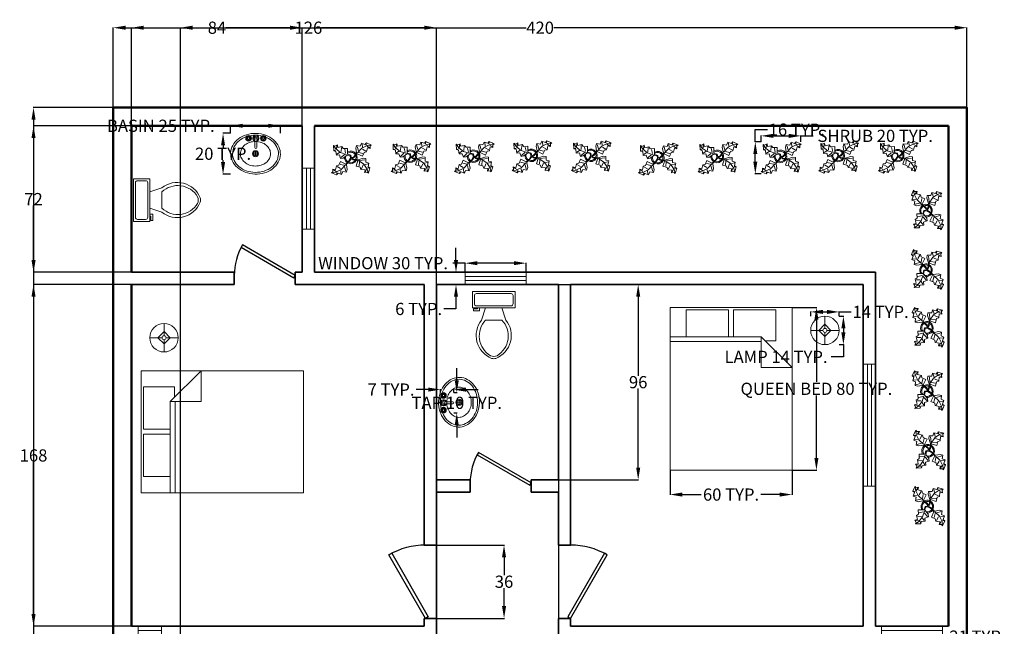
# Model space of a CAD drawing. Units: inches. Extents: x 823 to 1335, y 207 to 1074.
# Tile 6 of 6: x 823 to 1308, y 776 to 1074. Entities that reach past the tile are written whole.
import ezdxf

# ---------------------------------------------------------------- set-up
doc = ezdxf.new("R2010")
doc.units = ezdxf.units.IN
doc.header["$MEASUREMENT"] = 0
for name, color, linetype, lineweight in [('A-ANNO-DIMS', 2, 'Continuous', 18), ('doors', 51, 'Continuous', 25), ('furniture', 21, 'Continuous', 18), ('inner wall', 102, 'Continuous', 35), ('L-PLNT', 90, 'Continuous', 13), ('outer wall', 105, 'Continuous', 50), ('sanitary', 131, 'Continuous', 18), ('windows', 211, 'Continuous', 18)]:
    doc.layers.add(name, color=color, linetype=linetype, lineweight=lineweight)
doc.styles.get("Standard").update_dxf_attribs({"font": 'arial.ttf'})
doc.dimstyles.get("Standard").update_dxf_attribs({"dimtxt": 6, "dimasz": 6, "dimexe": 0.18, "dimexo": 0.0625, "dimgap": 0.09, "dimtad": 0, "dimtih": 1, "dimtoh": 1, "dimdec": 0, "dimzin": 0, "dimdsep": 46, "dimlunit": 3, "dimtxsty": 'Standard', "dimcen": 0.09, "dimadec": 0, "dimazin": 0, "dimtfac": 1, "dimtdec": 0, "dimtofl": 0, "dimtmove": 0, "dimatfit": 3, "dimfxl": 1, "dimtolj": 1, "dimtzin": 0, "dimarcsym": 0})

# ---------------------------------------------------------------- blocks, each defined once
blk = doc.blocks.new('*U3')
for p, q in [((0, 0), (0, 6)), ((40, 0), (40, 6))]:
    blk.add_line(p, q)
blk.add_lwpolyline([(0, 0), (34.64, -20), (35.52, -18.48), (0.87, 1.52)], close=True)
blk.add_arc((0, 0), 40, 330, 0)
blk = doc.blocks.new('*U2')
for p, q in [((0, 0), (0, -6)), ((40, 0), (40, -6))]:
    blk.add_line(p, q)
blk.add_lwpolyline([(0, 0), (34.64, 20), (35.52, 18.48), (0.87, -1.52)], close=True)
blk.add_arc((0, 0), 40, 0, 30)
blk = doc.blocks.new('*U5')
for p, q in [((0, 0), (0, -6)), ((-40, 0), (-40, -6))]:
    blk.add_line(p, q)
blk.add_lwpolyline([(0, 0), (-34.64, 20), (-35.52, 18.48), (-0.88, -1.52)], close=True)
blk.add_arc((0, 0), 40, 150, 180)
blk = doc.blocks.new('Bed - Queen')
for p, q in [((0, -80.00003), (0, 0)), ((0, 0), (59.99999, 0)), ((59.99999, 0), (59.99999, -80.00003)), ((7.99999, -1.2), (28.79998, -1.2)), ((7.99999, -14.4), (7.99999, -1.2)), ((28.79998, -1.2), (28.79998, -14.4)), ((31.19999, -1.2), (51.99999, -1.2)), ((31.19999, -14.4), (31.19999, -1.2)), ((51.99999, -1.2), (51.99999, -16.4)), ((0, -14.4), (44.8, -14.4)), ((59.99999, -29.6), (44.8, -14.4)), ((44.8, -14.4), (44.8, -29.6)), ((44.8, -16.8), (0, -16.8)), ((51.99999, -16.4), (46.79936, -16.4)), ((44.8, -29.6), (59.99999, -29.6)), ((59.99999, -80.00003), (0, -80.00003))]:
    blk.add_line(p, q)
blk = doc.blocks.new('Lamp - Table')
for p, q in [((0, 7), (0, 1)), ((-1, 0), (-7, 0)), ((0, 3), (-3, 0)), ((-3, 0), (0, -3)), ((3, 0), (0, 3)), ((0, -3), (3, 0)), ((1, 0), (7, 0)), ((0, -1), (0, -7))]:
    blk.add_line(p, q)
for radius in [7, 1]:
    blk.add_circle((0, 0), radius)
blk = doc.blocks.new('Sink - Oval top')
for p, q in [((-1, 0), (1, 0)), ((0, 1), (0, -1))]:
    blk.add_line(p, q)
for points in [[(-12.23, 0.39, 0.117634), (-11.46, -3.36, 0.104469), (-8.88, -6.8, 0.090016), (-5.08, -9.07, 0.08192), (-0.32, -10.02, 0.08192), (4.49, -9.38, 0.090016), (8.42, -7.36, 0.104469), (11.22, -4.09, 0.117634), (12.23, -0.39, 0.117634), (11.46, 3.36, 0.104469), (8.88, 6.8, 0.090016), (5.08, 9.07, 0.08192), (0.32, 10.02, 0.08192), (-4.49, 9.38, 0.090016), (-8.42, 7.36, 0.104469), (-11.22, 4.09, 0.117634)], [(-11.29, 0.16, 0.118622), (-10.52, -3.25, 0.104678), (-8.07, -6.36, 0.089562), (-4.54, -8.37, 0.081185), (-0.13, -9.15, 0.081185), (4.3, -8.49, 0.089562), (7.89, -6.58, 0.104678), (10.42, -3.55, 0.118622), (11.29, -0.16, 0.118622), (10.52, 3.25, 0.104678), (8.07, 6.36, 0.089562), (4.54, 8.37, 0.081185), (0.13, 9.15, 0.081185), (-4.3, 8.49, 0.089562), (-7.89, 6.58, 0.104678), (-10.42, 3.55, 0.118622)], [(-7.42, 0.08, 0.118283), (-6.91, -2.17, 0.104607), (-5.29, -4.21, 0.089718), (-2.97, -5.53, 0.081436), (-0.07, -6.04, 0.081436), (2.84, -5.59, 0.089718), (5.2, -4.33, 0.104607), (6.86, -2.32, 0.118283), (7.42, -0.08, 0.118283), (6.91, 2.17, 0.104607), (5.29, 4.21, 0.089718), (2.97, 5.53, 0.081436), (0.07, 6.04, 0.081436), (-2.84, 5.59, 0.089718), (-5.2, 4.33, 0.104607), (-6.86, 2.32, 0.118283)]]:
    blk.add_lwpolyline(points, format="xyb", close=True)
for radius in [1.5, 1]:
    blk.add_circle((0, 0), radius)
blk = doc.blocks.new('Faucet - Bathroom top')
for p, q in [((-4.107, 0.125), (-4.375, 0.125)), ((-3.75, 0.4788), (-3.75, 0.75)), ((-3.5, 0.482), (-3.5, 0.75)), ((-3.1461, 0.125), (-2.875, 0.125)), ((3.143, 0.125), (2.875, 0.125)), ((3.5, 0.4788), (3.5, 0.75)), ((3.75, 0.482), (3.75, 0.75)), ((4.1039, 0.125), (4.375, 0.125)), ((-4.1039, -0.125), (-4.375, -0.125)), ((-3.75, -0.4821), (-3.75, -0.75)), ((-3.5, -0.4789), (-3.5, -0.75)), ((-3.143, -0.125), (-2.875, -0.125)), ((-0.5, -0.8639), (-0.5, -4.5)), ((0.5, -4.5), (0.5, -0.8631)), ((3.1461, -0.125), (2.875, -0.125)), ((3.5, -0.4821), (3.5, -0.75)), ((3.75, -0.4789), (3.75, -0.75)), ((4.107, -0.125), (4.375, -0.125))]:
    blk.add_line(p, q)
for centre, radius in [((-3.625, 0), 1.375), ((-4.625, 0), 0.2795), ((-3.625, 0), 0.5), ((-3.625, 1), 0.2795), ((-2.625, 0), 0.2795), ((0, 0), 0.5), ((3.625, 0), 1.375), ((2.625, 0), 0.2795), ((3.625, 0), 0.5), ((3.625, 1), 0.2795), ((4.625, 0), 0.2795), ((-3.625, -1), 0.2795), ((3.625, -1), 0.2795)]:
    blk.add_circle(centre, radius)
for centre, radius, start, end in [((-3.625, 0), 1, 105.2407, 164.2093), ((-3.625, 0), 1, 16.44125, 74.07887), ((0, 0), 1.5, 289.6514, 250.3603), ((0, 0), 1, 300.3431, 239.7554), ((3.625, 0), 1, 106.12, 164.0884), ((3.625, 0), 1, 16.23422, 73.90469), ((-3.625, 0), 1, 196.2342, 253.9047), ((-3.625, 0), 1, 286.12, 344.0884), ((0, -4.5), 0.5, 180, 0), ((3.625, 0), 1, 196.4413, 254.0789), ((3.625, 0), 1, 285.2407, 344.2093)]:
    blk.add_arc(centre, radius, start, end)
blk = doc.blocks.new('Toilet - top')
for p, q in [((9.5, -6), (9.5, -2)), ((-10, -8.5), (-8, -8.5)), ((-10, -9.5), (-10, -8.5)), ((-7, -9.5), (-10, -9.5)), ((-8, -8.5), (-8, -8)), ((-7, -8), (-7, -9.5)), ((-4, -8), (-6, -14)), ((4, -8), (6, -14)), ((4, -14), (-4, -14))]:
    blk.add_line(p, q)
blk.add_lwpolyline([(10.5, -8), (10.5, 0), (-10.5, 0), (-10.5, -8)], close=True)
for points in [[(-9.5, -2), (-9.5, -6)], [(8.5, -1), (-8.5, -1)], [(-8.5, -7), (8.5, -7)]]:
    blk.add_lwpolyline(points)
for centre, radius, start, end in [((-8.62, -1.88), 0.884, 81.8699, 188.1301), ((8.62, -1.88), 0.884, 351.8699, 98.1301), ((-8.62, -6.12), 0.884, 171.8699, 278.1301), ((8.62, -6.12), 0.884, 261.8699, 8.1301), ((3.52, -21.58), 12.17, 141.4691, 247.9714), ((4.2, -21.82), 11.33, 136.3677, 238.9468), ((-3.52, -21.58), 12.17, 292.0284, 38.5307), ((-4.2, -21.82), 11.33, 301.053, 43.6321), ((0, -27.88), 4, 245.7318, 294.2682), ((0, -29), 4, 254.8605, 285.1395)]:
    blk.add_arc(centre, radius, start, end)
blk = doc.blocks.new('Plant - Rubber or Philodendron')
for p, q in [((-16.2005, 11.4774), (-13.9899, 8.1064)), ((-16.2005, 11.4774), (-14.8639, 10.7964)), ((-16.0159, 6.3329), (-16.2005, 11.4774)), ((-14.8639, 10.7964), (-12.6195, 11.8975)), ((-13.3174, 8.325), (-13.0735, 11.0065)), ((-12.6195, 11.8975), (-12.1909, 9.4345)), ((-12.1909, 9.4345), (-8.3829, 10.3)), ((-8.8369, 9.409), (-9.0894, 5.6095)), ((-8.3829, 10.3), (-7.0549, 8.501)), ((4.6914, 8.8812), (5.3859, 11.2828)), ((5.3859, 11.2828), (8.8871, 10.7908)), ((5.9878, 10.4842), (7.1971, 6.3869)), ((8.8871, 10.7908), (9.9809, 13.4933)), ((9.9809, 13.4933), (13.3837, 12.301)), ((15.3859, 11.3055), (10.3916, 8.7942)), ((10.5828, 12.6946), (10.8893, 9.7953)), ((13.3837, 12.301), (14.68, 13.9039)), ((14.5816, 13.2037), (14.3848, 11.8033)), ((14.68, 13.9039), (19.3848, 11.8146)), ((15.2875, 10.6053), (17.5907, 9.2105)), ((19.3848, 11.8146), (15.3859, 11.3055)), ((19.3848, 11.8146), (18.1868, 10.9119)), ((18.1868, 10.9119), (18.1925, 8.4119)), ((-14.0069, 5.8704), (-16.0159, 6.3329)), ((-15.3434, 6.5514), (-13.9984, 6.9884)), ((-13.5868, 2.2894), (-14.0069, 5.8704)), ((-13.9899, 8.1064), (-9.5434, 4.7185)), ((-10.6784, 2.491), (-13.5868, 2.2894)), ((-13.1329, 3.1804), (-10.6614, 4.727)), ((-9.5858, -0.8715), (-10.6784, 2.491)), ((-9.5434, 4.7185), (-4.1917, 2.9888)), ((-9.1318, 0.0195), (-5.9793, 2.9025)), ((-7.1228, -0.443), (-3.5248, 2.2131)), ((-7.0549, 8.501), (-3.0284, 8.6941)), ((-4.8529, 4.012), (-5.7184, 7.82)), ((-3.5248, 2.2131), (-3.3011, 2.4355)), ((-3.3011, 2.4355), (-0.5306, 1.7947)), ((-3.0284, 8.6941), (-3.0709, 3.1041)), ((-3.0709, 3.1041), (0.0797, 2.3163)), ((-0.5306, 1.7947), (-0.2255, -0.5527)), ((-0.5306, 1.7947), (-0.5306, 1.7947)), ((0.0797, 2.3163), (0.4866, -0.031)), ((0.4866, -0.031), (2.1141, 0.2298)), ((2.1141, 0.2298), (5.4346, 3.9146)), ((6.1032, 3.6844), (2.8262, -0.031)), ((4.6914, 8.8812), (5.5014, 4.4831)), ((5.4346, 3.9146), (5.5014, 4.4831)), ((11.1089, 1.1958), (6.1032, 3.6844)), ((10.3916, 8.7942), (6.2847, 4.4028)), ((7.7005, 4.8881), (11.5025, 3.9967)), ((14.2977, 6.1031), (10.9934, 7.9956)), ((12.7005, 4.8994), (11.1089, 1.1958)), ((14.8995, 5.3044), (12.7005, 4.8994)), ((15.7909, 9.1065), (14.8995, 5.3044)), ((18.1925, 8.4119), (15.7909, 9.1065)), ((-14.4141, -11.4699), (-13.5228, -7.6679)), ((-13.5228, -7.6679), (-11.3237, -7.2629)), ((-12.921, -8.4665), (-9.6166, -10.359)), ((-11.3237, -7.2629), (-9.7321, -3.5593)), ((-6.3237, -7.2516), (-10.1257, -6.3602)), ((-9.7321, -3.5593), (-4.7264, -6.0479)), ((-7.1228, -0.443), (-9.5858, -0.8715)), ((-9.0148, -11.1577), (-4.9047, -6.8122)), ((-4.611, -12.8477), (-5.8203, -8.7504)), ((-2.019, -3.6148), (-4.7264, -6.0479)), ((-4.1246, -6.8466), (-4.0579, -6.2781)), ((-3.3146, -11.2447), (-4.1246, -6.8466)), ((-4.0579, -6.2781), (-0.9375, -3.1608)), ((-2.019, -3.6148), (-0.2255, -0.5527)), ((-0.9375, -3.1608), (0.5883, -0.8135)), ((0.5883, -0.8135), (2.2447, -2.0916)), ((2.8262, -0.031), (1.3003, -0.5527)), ((1.3003, -0.5527), (2.4193, -1.4655)), ((2.2447, -2.0916), (6.7108, -2.6626)), ((2.4193, -1.4655), (6.895, -2.1175)), ((4.943, -7.9659), (6.7108, -2.6626)), ((8.8321, -9.0266), (4.943, -7.9659)), ((11.6605, -0.5413), (6.895, -2.1175)), ((12.3677, -6.1981), (7.219, -2.6772)), ((8.125, -4.0768), (7.7715, -7.9659)), ((8.3544, -2.7453), (13.1973, -2.1704)), ((9.5392, -11.1479), (8.8321, -9.0266)), ((10.2463, -10.4408), (11.6605, -6.9053)), ((11.6605, -0.5413), (14.1354, -0.8948)), ((15.5496, -10.7943), (12.3677, -6.1981)), ((16.2567, -5.8446), (13.4283, -6.5517)), ((14.1354, -0.8948), (14.1354, -4.4304)), ((14.1354, -4.4304), (16.9638, -5.1375)), ((16.9638, -5.1375), (16.2567, -8.673)), ((16.2567, -8.673), (18.0245, -9.7337)), ((-18.008, -14.1781), (-16.8101, -13.2754)), ((-18.008, -14.1781), (-14.0091, -13.669)), ((-13.3032, -16.2674), (-18.008, -14.1781)), ((-16.8157, -10.7754), (-14.4141, -11.4699)), ((-16.8101, -13.2754), (-16.8157, -10.7754)), ((-13.9107, -12.9688), (-16.2139, -11.574)), ((-14.0091, -13.669), (-9.0148, -11.1577)), ((-12.0069, -14.6645), (-13.3032, -16.2674)), ((-13.2048, -15.5672), (-13.008, -14.1668)), ((-8.6042, -15.8568), (-12.0069, -14.6645)), ((-9.206, -15.0581), (-9.5126, -12.1588)), ((-7.5103, -13.1543), (-8.6042, -15.8568)), ((-4.0092, -13.6463), (-7.5103, -13.1543)), ((-3.3146, -11.2447), (-4.0092, -13.6463)), ((13.4283, -11.5015), (9.5392, -11.1479)), ((13.0748, -13.9763), (13.4283, -11.5015)), ((15.5496, -13.6228), (13.0748, -13.9763)), ((14.8425, -10.7943), (13.7819, -13.2692)), ((16.6103, -14.6834), (15.5496, -10.7943)), ((16.6103, -14.6834), (15.5496, -13.6228)), ((17.3174, -9.7337), (15.9032, -9.7337)), ((18.0245, -9.7337), (16.6103, -14.6834))]:
    blk.add_line(p, q)
for centre, radius, start, end in [((0.0308, 0.1664), 6, 178.6147, 235.1169), ((0.0308, 0.1664), 5, 168.1647, 238.6725), ((0, 0), 6.1275, 34.37569, 120.1028), ((-0.0601, -0.2075), 5.2461, 33.82192, 124.9414), ((-0.2664, 0.1682), 5.2775, 338.4094, 20.03007), ((-0.098, 0.1364), 6.1288, 341.2017, 26.09184), ((-0.0234, 0.3825), 6.1492, 242.5812, 331.2714), ((-0.1102, 0.4886), 5.2883, 247.3711, 327.472)]:
    blk.add_arc(centre, radius, start, end)
blk = doc.blocks.new('WIN-60IN')
for p, q in [((0, 0), (0, 60)), ((0, 60), (6, 60)), ((2, 0), (2, 60)), ((4, 60), (4, 0)), ((6, 60), (6, 0)), ((6, 0), (0, 0))]:
    blk.add_line(p, q)
blk = doc.blocks.new('WIN-30IN')
for p, q in [((0, 6), (30, 6)), ((0, 0), (0, 6)), ((30, 6), (30, 0)), ((0, 4), (30, 4)), ((30, 2), (0, 2)), ((30, 0), (0, 0))]:
    blk.add_line(p, q)
blk = doc.blocks.new('WIN-LIGHTWELL-NARROW')
for p, q in [((0, 6), (0, 0)), ((11.5, 6), (11.5, 0)), ((0, 4), (11.5, 4)), ((0, 2), (11.5, 2))]:
    blk.add_line(p, q)
blk = doc.blocks.new('*D26')
at = {"layer": 'A-ANNO-DIMS', "color": 0, "lineweight": -2, "transparency": 16777216}
for p, q in [((1203.26, 932.36), (1215.38, 932.36)), ((1215.2, 926.36), (1215.2, 895.74)), ((1215.2, 858.36), (1215.2, 888.99)), ((1203.26, 852.36), (1215.38, 852.36))]:
    blk.add_line(p, q, dxfattribs=at)
for points in [[(1214.2, 926.36), (1216.2, 926.36), (1215.2, 932.36)], [(1214.2, 858.36), (1216.2, 858.36), (1215.2, 852.36)]]:
    blk.add_solid(points, dxfattribs=at)
at = {"layer": 'Defpoints', "color": 0, "lineweight": -2, "transparency": 16777216}
for p in [(1203.2, 932.36), (1215.2, 932.36), (1203.2, 852.36)]:
    blk.add_point(p, dxfattribs=at)
at = {"layer": 'A-ANNO-DIMS', "color": 0, "transparency": 16777216, "insert": (1215.2, 892.36), "char_height": 6, "attachment_point": 5}
blk.add_mtext('\\A1;QUEEN BED 80 TYP.', dxfattribs=at)
blk = doc.blocks.new('*D27')
at = {"layer": 'A-ANNO-DIMS', "color": 0, "lineweight": -2, "transparency": 16777216}
for p, q in [((1143.2, 852.3), (1143.2, 840.18)), ((1203.2, 852.3), (1203.2, 840.18)), ((1149.2, 840.36), (1158.49, 840.36)), ((1197.2, 840.36), (1187.91, 840.36))]:
    blk.add_line(p, q, dxfattribs=at)
for points in [[(1149.2, 841.36), (1149.2, 839.36), (1143.2, 840.36)], [(1197.2, 841.36), (1197.2, 839.36), (1203.2, 840.36)]]:
    blk.add_solid(points, dxfattribs=at)
at = {"layer": 'Defpoints', "color": 0, "lineweight": -2, "transparency": 16777216}
for p in [(1143.2, 852.36), (1203.2, 852.36), (1203.2, 840.36)]:
    blk.add_point(p, dxfattribs=at)
at = {"layer": 'A-ANNO-DIMS', "color": 0, "transparency": 16777216, "insert": (1173.2, 840.36), "char_height": 6, "attachment_point": 5}
blk.add_mtext('\\A1;60 TYP.', dxfattribs=at)
blk = doc.blocks.new('*D28')
at = {"layer": 'A-ANNO-DIMS', "color": 0, "lineweight": -2, "transparency": 16777216}
for p, q in [((1226.44, 928.05), (1228.66, 928.05)), ((1228.48, 922.05), (1228.48, 920.05)), ((1226.44, 914.05), (1228.66, 914.05)), ((1228.48, 914.05), (1228.48, 908.05)), ((1228.48, 908.05), (1222.48, 908.05))]:
    blk.add_line(p, q, dxfattribs=at)
for points in [[(1227.48, 922.05), (1229.48, 922.05), (1228.48, 928.05)], [(1227.48, 920.05), (1229.48, 920.05), (1228.48, 914.05)]]:
    blk.add_solid(points, dxfattribs=at)
at = {"layer": 'Defpoints', "color": 0, "lineweight": -2, "transparency": 16777216}
for p in [(1226.38, 928.05), (1226.38, 914.05), (1228.48, 914.05)]:
    blk.add_point(p, dxfattribs=at)
at = {"layer": 'A-ANNO-DIMS', "color": 0, "transparency": 16777216, "insert": (1195.34, 908.05), "char_height": 6, "attachment_point": 5}
blk.add_mtext('\\A1;LAMP 14 TYP.', dxfattribs=at)
blk = doc.blocks.new('*D29')
at = {"layer": 'A-ANNO-DIMS', "color": 0, "lineweight": -2, "transparency": 16777216}
for p, q in [((1212.38, 928.11), (1212.38, 930.33)), ((1226.38, 928.11), (1226.38, 930.33)), ((1218.38, 930.15), (1220.38, 930.15)), ((1226.38, 930.15), (1232.38, 930.15))]:
    blk.add_line(p, q, dxfattribs=at)
for points in [[(1218.38, 931.15), (1218.38, 929.15), (1212.38, 930.15)], [(1220.38, 931.15), (1220.38, 929.15), (1226.38, 930.15)]]:
    blk.add_solid(points, dxfattribs=at)
at = {"layer": 'Defpoints', "color": 0, "lineweight": -2, "transparency": 16777216}
for p in [(1212.38, 928.05), (1226.38, 930.15), (1226.38, 928.05)]:
    blk.add_point(p, dxfattribs=at)
at = {"layer": 'A-ANNO-DIMS', "color": 0, "transparency": 16777216, "insert": (1246.79, 930.15), "char_height": 6, "attachment_point": 5}
blk.add_mtext('\\A1;14 TYP.', dxfattribs=at)
blk = doc.blocks.new('*D40')
at = {"layer": 'A-ANNO-DIMS', "color": 0, "lineweight": -2, "transparency": 16777216}
for p, q in [((926.94, 1021.65), (920.94, 1021.65)), ((926.94, 1018.03), (926.94, 1021.83)), ((945.49, 1021.65), (932.94, 1021.65)), ((951.49, 1018.03), (951.49, 1021.83))]:
    blk.add_line(p, q, dxfattribs=at)
for points in [[(932.94, 1022.65), (932.94, 1020.65), (926.94, 1021.65)], [(945.49, 1022.65), (945.49, 1020.65), (951.49, 1021.65)]]:
    blk.add_solid(points, dxfattribs=at)
at = {"layer": 'Defpoints', "color": 0, "lineweight": -2, "transparency": 16777216}
for p in [(926.94, 1021.65), (926.94, 1017.97), (951.49, 1017.97)]:
    blk.add_point(p, dxfattribs=at)
at = {"layer": 'A-ANNO-DIMS', "color": 0, "transparency": 16777216, "insert": (892.64, 1021.65), "char_height": 6, "attachment_point": 5}
blk.add_mtext('\\A1;BASIN 25 TYP.', dxfattribs=at)
blk = doc.blocks.new('*D41')
at = {"layer": 'A-ANNO-DIMS', "color": 0, "lineweight": -2, "transparency": 16777216}
for p, q in [((926.88, 1017.97), (923.08, 1017.97)), ((923.26, 1011.97), (923.26, 1011.05)), ((923.26, 1003.83), (923.26, 1004.74)), ((926.88, 997.83), (923.08, 997.83))]:
    blk.add_line(p, q, dxfattribs=at)
for points in [[(922.26, 1011.97), (924.26, 1011.97), (923.26, 1017.97)], [(922.26, 1003.83), (924.26, 1003.83), (923.26, 997.83)]]:
    blk.add_solid(points, dxfattribs=at)
at = {"layer": 'Defpoints', "color": 0, "lineweight": -2, "transparency": 16777216}
for p in [(926.94, 1017.97), (923.26, 997.83), (926.94, 997.83)]:
    blk.add_point(p, dxfattribs=at)
at = {"layer": 'A-ANNO-DIMS', "color": 0, "transparency": 16777216, "insert": (923.26, 1007.9), "char_height": 6, "attachment_point": 5}
blk.add_mtext('\\A1;20 TYP.', dxfattribs=at)
blk = doc.blocks.new('*D42')
at = {"layer": 'A-ANNO-DIMS', "color": 0, "lineweight": -2, "transparency": 16777216}
for p, q in [((1038.24, 896.46), (1038.24, 902.46)), ((1036.8, 890.46), (1038.42, 890.46)), ((1036.8, 880.46), (1038.42, 880.46)), ((1038.24, 874.46), (1038.24, 868.46))]:
    blk.add_line(p, q, dxfattribs=at)
for points in [[(1037.24, 896.46), (1039.24, 896.46), (1038.24, 890.46)], [(1037.24, 874.46), (1039.24, 874.46), (1038.24, 880.46)]]:
    blk.add_solid(points, dxfattribs=at)
at = {"layer": 'Defpoints', "color": 0, "lineweight": -2, "transparency": 16777216}
for p in [(1036.74, 890.46), (1038.24, 890.46), (1036.74, 880.46)]:
    blk.add_point(p, dxfattribs=at)
at = {"layer": 'A-ANNO-DIMS', "color": 0, "transparency": 16777216, "insert": (1038.24, 885.46), "char_height": 6, "attachment_point": 5}
blk.add_mtext('\\A1;TAP 10 TYP.', dxfattribs=at)
blk = doc.blocks.new('*D43')
at = {"layer": 'A-ANNO-DIMS', "color": 0, "lineweight": -2, "transparency": 16777216}
for p, q in [((1024.24, 891.96), (1018.24, 891.96)), ((1030.24, 890.53), (1030.24, 892.14)), ((1036.74, 890.53), (1036.74, 892.14)), ((1042.74, 891.96), (1048.74, 891.96))]:
    blk.add_line(p, q, dxfattribs=at)
for points in [[(1024.24, 892.96), (1024.24, 890.96), (1030.24, 891.96)], [(1042.74, 892.96), (1042.74, 890.96), (1036.74, 891.96)]]:
    blk.add_solid(points, dxfattribs=at)
at = {"layer": 'Defpoints', "color": 0, "lineweight": -2, "transparency": 16777216}
for p in [(1030.24, 891.96), (1030.24, 890.46), (1036.74, 890.46)]:
    blk.add_point(p, dxfattribs=at)
at = {"layer": 'A-ANNO-DIMS', "color": 0, "transparency": 16777216, "insert": (1005.9, 891.96), "char_height": 6, "attachment_point": 5}
blk.add_mtext('\\A1;7 TYP.', dxfattribs=at)
blk = doc.blocks.new('*D45')
at = {"layer": 'A-ANNO-DIMS', "color": 0, "lineweight": -2, "transparency": 16777216}
for p, q in [((1252.69, 765.63), (1252.69, 770.71)), ((1258.69, 770.53), (1267.69, 770.53)), ((1273.69, 765.63), (1273.69, 770.71)), ((1273.69, 770.53), (1279.69, 770.53))]:
    blk.add_line(p, q, dxfattribs=at)
for points in [[(1258.69, 771.53), (1258.69, 769.53), (1252.69, 770.53)], [(1267.69, 771.53), (1267.69, 769.53), (1273.69, 770.53)]]:
    blk.add_solid(points, dxfattribs=at)
at = {"layer": 'Defpoints', "color": 0, "lineweight": -2, "transparency": 16777216}
for p in [(1273.69, 770.53), (1252.69, 765.57), (1273.69, 765.57)]:
    blk.add_point(p, dxfattribs=at)
at = {"layer": 'A-ANNO-DIMS', "color": 0, "transparency": 16777216, "insert": (1294.44, 770.53), "char_height": 6, "attachment_point": 5}
blk.add_mtext('\\A1;21 TYP.', dxfattribs=at)
blk = doc.blocks.new('*D48')
at = {"layer": 'A-ANNO-DIMS', "color": 0, "lineweight": -2, "transparency": 16777216}
for p, q in [((1042.37, 954.11), (1036.37, 954.11)), ((1042.37, 949.67), (1042.37, 954.29)), ((1066.37, 954.11), (1048.37, 954.11)), ((1072.37, 949.67), (1072.37, 954.29))]:
    blk.add_line(p, q, dxfattribs=at)
for points in [[(1048.37, 955.11), (1048.37, 953.11), (1042.37, 954.11)], [(1066.37, 955.11), (1066.37, 953.11), (1072.37, 954.11)]]:
    blk.add_solid(points, dxfattribs=at)
at = {"layer": 'Defpoints', "color": 0, "lineweight": -2, "transparency": 16777216}
for p in [(1042.37, 954.11), (1042.37, 949.61), (1072.37, 949.61)]:
    blk.add_point(p, dxfattribs=at)
at = {"layer": 'A-ANNO-DIMS', "color": 0, "transparency": 16777216, "insert": (1002, 954.11), "char_height": 6, "attachment_point": 5}
blk.add_mtext('\\A1;WINDOW 30 TYP.', dxfattribs=at)
blk = doc.blocks.new('*D49')
at = {"layer": 'A-ANNO-DIMS', "color": 0, "lineweight": -2, "transparency": 16777216}
for p, q in [((1037.87, 955.61), (1037.87, 961.61)), ((1042.3, 949.61), (1037.69, 949.61)), ((1042.3, 943.61), (1037.69, 943.61)), ((1037.87, 937.61), (1037.87, 931.61)), ((1037.87, 931.61), (1031.87, 931.61))]:
    blk.add_line(p, q, dxfattribs=at)
for points in [[(1036.87, 955.61), (1038.87, 955.61), (1037.87, 949.61)], [(1036.87, 937.61), (1038.87, 937.61), (1037.87, 943.61)]]:
    blk.add_solid(points, dxfattribs=at)
at = {"layer": 'Defpoints', "color": 0, "lineweight": -2, "transparency": 16777216}
for p in [(1042.37, 949.61), (1037.87, 943.61), (1042.37, 943.61)]:
    blk.add_point(p, dxfattribs=at)
at = {"layer": 'A-ANNO-DIMS', "color": 0, "transparency": 16777216, "insert": (1019.49, 931.61), "char_height": 6, "attachment_point": 5}
blk.add_mtext('\\A1;6 TYP.', dxfattribs=at)
blk = doc.blocks.new('*D52')
at = {"layer": 'A-ANNO-DIMS', "color": 0, "lineweight": -2, "transparency": 16777216}
for p, q in [((1188.07, 1013.82), (1188.07, 1016.87)), ((1194.07, 1016.69), (1201.62, 1016.69)), ((1207.62, 1013.82), (1207.62, 1016.87)), ((1207.62, 1016.69), (1213.62, 1016.69))]:
    blk.add_line(p, q, dxfattribs=at)
for points in [[(1194.07, 1017.69), (1194.07, 1015.69), (1188.07, 1016.69)], [(1201.62, 1017.69), (1201.62, 1015.69), (1207.62, 1016.69)]]:
    blk.add_solid(points, dxfattribs=at)
at = {"layer": 'Defpoints', "color": 0, "lineweight": -2, "transparency": 16777216}
for p in [(1188.07, 1013.76), (1207.62, 1016.69), (1207.62, 1013.76)]:
    blk.add_point(p, dxfattribs=at)
at = {"layer": 'A-ANNO-DIMS', "color": 0, "transparency": 16777216, "insert": (1244.13, 1016.69), "char_height": 6, "attachment_point": 5}
blk.add_mtext('\\A1;SHRUB 20 TYP.', dxfattribs=at)
blk = doc.blocks.new('*D53')
at = {"layer": 'A-ANNO-DIMS', "color": 0, "lineweight": -2, "transparency": 16777216}
for p, q in [((1185.14, 1013.76), (1185.14, 1019.76)), ((1185.14, 1019.76), (1191.14, 1019.76)), ((1188.01, 1013.76), (1184.96, 1013.76)), ((1185.14, 1003.99), (1185.14, 1007.76)), ((1188.01, 997.99), (1184.96, 997.99))]:
    blk.add_line(p, q, dxfattribs=at)
for points in [[(1184.14, 1007.76), (1186.14, 1007.76), (1185.14, 1013.76)], [(1184.14, 1003.99), (1186.14, 1003.99), (1185.14, 997.99)]]:
    blk.add_solid(points, dxfattribs=at)
at = {"layer": 'Defpoints', "color": 0, "lineweight": -2, "transparency": 16777216}
for p in [(1185.14, 1013.76), (1188.07, 1013.76), (1188.07, 997.99)]:
    blk.add_point(p, dxfattribs=at)
at = {"layer": 'A-ANNO-DIMS', "color": 0, "transparency": 16777216, "insert": (1205.55, 1019.76), "char_height": 6, "attachment_point": 5}
blk.add_mtext('\\A1;16 TYP.', dxfattribs=at)
blk = doc.blocks.new('*D56')
at = {"layer": 'A-ANNO-DIMS', "color": 0, "lineweight": -2, "transparency": 16777216}
for p, q in [((869.26, 1030.67), (869.26, 1070.04)), ((875.26, 1069.86), (1072.43, 1069.86)), ((1283.26, 1069.86), (1086.09, 1069.86)), ((1289.26, 1030.67), (1289.26, 1070.04))]:
    blk.add_line(p, q, dxfattribs=at)
for points in [[(875.26, 1070.86), (875.26, 1068.86), (869.26, 1069.86)], [(1283.26, 1070.86), (1283.26, 1068.86), (1289.26, 1069.86)]]:
    blk.add_solid(points, dxfattribs=at)
at = {"layer": 'Defpoints', "color": 0, "lineweight": -2, "transparency": 16777216}
for p in [(1289.26, 1069.86), (869.26, 1030.61), (1289.26, 1030.61)]:
    blk.add_point(p, dxfattribs=at)
at = {"layer": 'A-ANNO-DIMS', "color": 0, "transparency": 16777216, "insert": (1079.26, 1069.86), "char_height": 6, "attachment_point": 5}
blk.add_mtext('\\A1;420', dxfattribs=at)
blk = doc.blocks.new('*D57')
at = {"layer": 'A-ANNO-DIMS', "color": 0, "lineweight": -2, "transparency": 16777216}
for p, q in [((869.2, 1030.61), (829.83, 1030.61)), ((830.01, 1024.61), (830.01, 643.76)), ((830.01, 256.61), (830.01, 637.45)), ((869.2, 250.61), (829.83, 250.61))]:
    blk.add_line(p, q, dxfattribs=at)
for points in [[(829.01, 1024.61), (831.01, 1024.61), (830.01, 1030.61)], [(829.01, 256.61), (831.01, 256.61), (830.01, 250.61)]]:
    blk.add_solid(points, dxfattribs=at)
at = {"layer": 'Defpoints', "color": 0, "lineweight": -2, "transparency": 16777216}
for p in [(830.01, 1030.61), (869.26, 1030.61), (869.26, 250.61)]:
    blk.add_point(p, dxfattribs=at)
at = {"layer": 'A-ANNO-DIMS', "color": 0, "transparency": 16777216, "insert": (830.01, 640.61), "char_height": 6, "attachment_point": 5}
blk.add_mtext('\\A1;780', dxfattribs=at)
blk = doc.blocks.new('*D58')
at = {"layer": 'A-ANNO-DIMS', "color": 0, "lineweight": -2, "transparency": 16777216}
for p, q in [((878.26, 1021.67), (878.26, 1070.04)), ((884.26, 1069.86), (915.88, 1069.86)), ((956.26, 1069.86), (924.64, 1069.86)), ((962.26, 1021.67), (962.26, 1070.04))]:
    blk.add_line(p, q, dxfattribs=at)
for points in [[(884.26, 1070.86), (884.26, 1068.86), (878.26, 1069.86)], [(956.26, 1070.86), (956.26, 1068.86), (962.26, 1069.86)]]:
    blk.add_solid(points, dxfattribs=at)
at = {"layer": 'Defpoints', "color": 0, "lineweight": -2, "transparency": 16777216}
for p in [(962.26, 1069.86), (878.26, 1021.61), (962.26, 1021.61)]:
    blk.add_point(p, dxfattribs=at)
at = {"layer": 'A-ANNO-DIMS', "color": 0, "transparency": 16777216, "insert": (920.26, 1069.86), "char_height": 6, "attachment_point": 5}
blk.add_mtext('\\A1;84', dxfattribs=at)
blk = doc.blocks.new('*D59')
at = {"layer": 'A-ANNO-DIMS', "color": 0, "lineweight": -2, "transparency": 16777216}
for p, q in [((878.2, 1021.61), (829.83, 1021.61)), ((830.01, 1015.61), (830.01, 988.71)), ((830.01, 955.61), (830.01, 982.5)), ((878.2, 949.61), (829.83, 949.61))]:
    blk.add_line(p, q, dxfattribs=at)
for points in [[(829.01, 1015.61), (831.01, 1015.61), (830.01, 1021.61)], [(829.01, 955.61), (831.01, 955.61), (830.01, 949.61)]]:
    blk.add_solid(points, dxfattribs=at)
at = {"layer": 'Defpoints', "color": 0, "lineweight": -2, "transparency": 16777216}
for p in [(878.26, 1021.61), (830.01, 949.61), (878.26, 949.61)]:
    blk.add_point(p, dxfattribs=at)
at = {"layer": 'A-ANNO-DIMS', "color": 0, "transparency": 16777216, "insert": (830.01, 985.61), "char_height": 6, "attachment_point": 5}
blk.add_mtext('\\A1;72', dxfattribs=at)
blk = doc.blocks.new('*D61')
at = {"layer": 'A-ANNO-DIMS', "color": 0, "lineweight": -2, "transparency": 16777216}
for p, q in [((1028.26, 847.54), (1028.26, 211.18)), ((1088.26, 847.54), (1088.26, 211.18)), ((1034.26, 211.36), (1053.87, 211.36)), ((1082.26, 211.36), (1062.66, 211.36))]:
    blk.add_line(p, q, dxfattribs=at)
for points in [[(1034.26, 212.36), (1034.26, 210.36), (1028.26, 211.36)], [(1082.26, 212.36), (1082.26, 210.36), (1088.26, 211.36)]]:
    blk.add_solid(points, dxfattribs=at)
at = {"layer": 'Defpoints', "color": 0, "lineweight": -2, "transparency": 16777216}
for p in [(1028.26, 847.61), (1088.26, 847.61), (1088.26, 211.36)]:
    blk.add_point(p, dxfattribs=at)
at = {"layer": 'A-ANNO-DIMS', "color": 0, "transparency": 16777216, "insert": (1058.26, 211.36), "char_height": 6, "attachment_point": 5}
blk.add_mtext('\\A1;60', dxfattribs=at)
blk = doc.blocks.new('*D63')
at = {"layer": 'A-ANNO-DIMS', "color": 0, "lineweight": -2, "transparency": 16777216}
for p, q in [((878.2, 943.61), (829.83, 943.61)), ((830.01, 937.61), (830.01, 862.76)), ((830.01, 781.61), (830.01, 856.45)), ((878.2, 775.61), (829.83, 775.61))]:
    blk.add_line(p, q, dxfattribs=at)
for points in [[(829.01, 937.61), (831.01, 937.61), (830.01, 943.61)], [(829.01, 781.61), (831.01, 781.61), (830.01, 775.61)]]:
    blk.add_solid(points, dxfattribs=at)
at = {"layer": 'Defpoints', "color": 0, "lineweight": -2, "transparency": 16777216}
for p in [(830.01, 943.61), (878.26, 943.61), (878.26, 775.61)]:
    blk.add_point(p, dxfattribs=at)
at = {"layer": 'A-ANNO-DIMS', "color": 0, "transparency": 16777216, "insert": (830.01, 859.61), "char_height": 6, "attachment_point": 5}
blk.add_mtext('\\A1;168', dxfattribs=at)
blk = doc.blocks.new('*D64')
at = {"layer": 'A-ANNO-DIMS', "color": 0, "lineweight": -2, "transparency": 16777216}
for p, q in [((1088.32, 943.61), (1127.69, 943.61)), ((1127.51, 937.61), (1127.51, 898.76)), ((1127.51, 853.61), (1127.51, 892.45)), ((1088.32, 847.61), (1127.69, 847.61))]:
    blk.add_line(p, q, dxfattribs=at)
for points in [[(1126.51, 937.61), (1128.51, 937.61), (1127.51, 943.61)], [(1126.51, 853.61), (1128.51, 853.61), (1127.51, 847.61)]]:
    blk.add_solid(points, dxfattribs=at)
at = {"layer": 'Defpoints', "color": 0, "lineweight": -2, "transparency": 16777216}
for p in [(1088.26, 943.61), (1088.26, 847.61), (1127.51, 847.61)]:
    blk.add_point(p, dxfattribs=at)
at = {"layer": 'A-ANNO-DIMS', "color": 0, "transparency": 16777216, "insert": (1127.51, 895.61), "char_height": 6, "attachment_point": 5}
blk.add_mtext('\\A1;96', dxfattribs=at)
blk = doc.blocks.new('*D66')
at = {"layer": 'A-ANNO-DIMS', "color": 0, "lineweight": -2, "transparency": 16777216}
for p, q in [((902.26, 769.67), (902.26, 1070.04)), ((908.26, 1069.86), (958.83, 1069.86)), ((1022.26, 1069.86), (971.7, 1069.86)), ((1028.26, 769.67), (1028.26, 1070.04))]:
    blk.add_line(p, q, dxfattribs=at)
for points in [[(908.26, 1070.86), (908.26, 1068.86), (902.26, 1069.86)], [(1022.26, 1070.86), (1022.26, 1068.86), (1028.26, 1069.86)]]:
    blk.add_solid(points, dxfattribs=at)
at = {"layer": 'Defpoints', "color": 0, "lineweight": -2, "transparency": 16777216}
for p in [(1028.26, 1069.86), (902.26, 769.61), (1028.26, 769.61)]:
    blk.add_point(p, dxfattribs=at)
at = {"layer": 'A-ANNO-DIMS', "color": 0, "transparency": 16777216, "insert": (965.26, 1069.86), "char_height": 6, "attachment_point": 5}
blk.add_mtext('\\A1;126', dxfattribs=at)
blk = doc.blocks.new('*D82')
at = {"layer": 'A-ANNO-DIMS', "color": 0, "lineweight": -2, "transparency": 16777216}
for p, q in [((1022.32, 815.51), (1061.69, 815.51)), ((1061.51, 809.51), (1061.51, 800.67)), ((1061.51, 785.51), (1061.51, 794.36)), ((1022.32, 779.51), (1061.69, 779.51))]:
    blk.add_line(p, q, dxfattribs=at)
for points in [[(1060.51, 809.51), (1062.51, 809.51), (1061.51, 815.51)], [(1060.51, 785.51), (1062.51, 785.51), (1061.51, 779.51)]]:
    blk.add_solid(points, dxfattribs=at)
at = {"layer": 'Defpoints', "color": 0, "lineweight": -2, "transparency": 16777216}
for p in [(1022.26, 815.51), (1022.26, 779.51), (1061.51, 779.51)]:
    blk.add_point(p, dxfattribs=at)
at = {"layer": 'A-ANNO-DIMS', "color": 0, "transparency": 16777216, "insert": (1061.51, 797.51), "char_height": 6, "attachment_point": 5}
blk.add_mtext('\\A1;36', dxfattribs=at)

msp = doc.modelspace()

# ---------------------------------------------------------------- linework, layer by layer
at = {"layer": 'inner wall'}
for p, q in [((962.26, 949.61), (962.26, 1021.61)), ((968.26, 949.61), (968.26, 1021.61)), ((878.26, 949.61), (928.79, 949.61)), ((958.79, 949.61), (962.26, 949.61)), ((968.26, 949.61), (1244.26, 949.61)), ((1244.26, 949.61), (1244.26, 775.61)), ((878.26, 943.61), (928.79, 943.61)), ((958.79, 943.61), (1022.26, 943.61)), ((1022.26, 815.51), (1022.26, 943.61)), ((1022.26, 815.51), (1022.26, 943.61)), ((1028.26, 943.61), (1088.26, 943.61)), ((1028.26, 943.61), (1088.26, 943.61)), ((1028.26, 847.61), (1028.26, 943.61)), ((1088.26, 943.61), (1088.26, 847.61)), ((1094.26, 943.61), (1094.26, 815.51)), ((1094.26, 943.61), (1238.26, 943.61)), ((1238.26, 943.61), (1238.26, 775.61)), ((1028.26, 847.61), (1044.85, 847.61)), ((1074.85, 847.61), (1088.26, 847.61)), ((1028.26, 841.61), (1044.85, 841.61)), ((1028.26, 815.51), (1028.26, 841.61)), ((1074.85, 841.61), (1088.26, 841.61)), ((1088.26, 841.61), (1088.26, 815.51)), ((878.26, 775.61), (1022.26, 775.61)), ((1022.26, 775.61), (1022.26, 779.51)), ((1022.26, 775.61), (1022.26, 779.51)), ((1028.26, 769.61), (1028.26, 779.51)), ((1088.26, 779.51), (1088.26, 759.05)), ((1094.26, 779.51), (1094.26, 775.61)), ((1094.26, 775.61), (1238.26, 775.61)), ((1244.26, 775.61), (1280.26, 775.61))]:
    msp.add_line(p, q, dxfattribs=at)
for points in [[(928.79, 943.61), (928.79, 949.61)], [(958.79, 949.61), (958.79, 943.61)], [(1044.85, 841.61), (1044.85, 847.61)], [(1074.85, 847.61), (1074.85, 841.61)], [(1028.26, 815.51), (1022.26, 815.51)], [(1094.26, 815.51), (1088.26, 815.51)], [(1022.26, 779.51), (1028.26, 779.51)], [(1088.26, 779.51), (1094.26, 779.51)]]:
    msp.add_lwpolyline(points, dxfattribs=at)
at = {"layer": 'outer wall'}
for p, q in [((878.26, 1021.61), (962.26, 1021.61)), ((878.26, 949.61), (878.26, 1021.61)), ((968.26, 1021.61), (1280.26, 1021.61)), ((1280.26, 775.61), (1280.26, 1021.61)), ((878.26, 775.61), (878.26, 943.61))]:
    msp.add_line(p, q, dxfattribs=at)
msp.add_lwpolyline([(869.26, 1030.61), (1289.26, 1030.61), (1289.26, 250.61), (869.26, 250.61)], close=True, dxfattribs=at)

# ---------------------------------------------------------------- block references
at = {"layer": 'doors', "xscale": 0.75, "yscale": 0.75, "zscale": 0.75}
for p in [(958.79, 948.11), (1074.85, 846.11)]:
    msp.add_blockref('*U5', p, dxfattribs=at)
at = {"layer": 'doors', "xscale": 0.9, "yscale": 0.9, "zscale": 0.9, "rotation": 90}
for name, p in [('*U2', (1022.86, 779.51)), ('*U3', (1094.26, 779.51))]:
    msp.add_blockref(name, p, dxfattribs=at)
at = {"layer": 'furniture'}
for name, p in [('Bed - Queen', (1143.2, 932.36)), ('Lamp - Table', (894.22, 917.45))]:
    msp.add_blockref(name, p, dxfattribs=at)
for name, p, rotation in [('Lamp - Table', (1219.38, 921.05), 270), ('Bed - Queen', (882.91, 841.26), 90)]:
    msp.add_blockref(name, p, dxfattribs=dict(at, rotation=rotation))
at = {"layer": 'L-PLNT', "xscale": 0.5226467583176748, "yscale": 0.5226467583176748, "zscale": 0.5226467583176748}
for p in [(986.1, 1006.01), (1015.38, 1006.62), (1046.5, 1006.62), (1074.87, 1007.03), (1104.15, 1007.03), (1137.09, 1005.88), (1166.37, 1006.49), (1197.49, 1006.49), (1225.86, 1006.9), (1255.14, 1006.9)]:
    msp.add_blockref('Plant - Rubber or Philodendron', p, dxfattribs=at)
at = {"layer": 'L-PLNT', "xscale": 0.5226467583176748, "yscale": 0.5226467583176748, "zscale": 0.5226467583176748, "rotation": 90}
for p in [(1269.23, 979.91), (1269.23, 950.62), (1269.64, 922.25), (1269.64, 891.13), (1270.25, 861.85), (1269.89, 834.41)]:
    msp.add_blockref('Plant - Rubber or Philodendron', p, dxfattribs=at)
at = {"layer": 'sanitary'}
for name, p, rotation in [('Sink - Oval top', (939.22, 1007.9), 180), ('Toilet - top', (879.17, 985.14), 90), ('Sink - Oval top', (1039.35, 885.74), 89.99999999999996), ('Faucet - Bathroom top', (1031.74, 885.46), 90)]:
    msp.add_blockref(name, p, dxfattribs=dict(at, rotation=rotation))
for name, p in [('Faucet - Bathroom top', (939.43, 1015.51)), ('Toilet - top', (1056.45, 940.16))]:
    msp.add_blockref(name, p, dxfattribs=at)
at = {"layer": 'windows'}
for p, rotation in [((962.26, 1000.78), 270.0000000000002), ((1072.37, 949.61), 180)]:
    msp.add_blockref('WIN-30IN', p, dxfattribs=dict(at, rotation=rotation))
for name, p in [('WIN-60IN', (1238.26, 844.52)), ('WIN-LIGHTWELL-NARROW', (881.44, 769.61)), ('WIN-30IN', (1247.3, 769.61))]:
    msp.add_blockref(name, p, dxfattribs=at)

# ---------------------------------------------------------------- dimensions: what is measured, and where the dimension line sits
at = {"layer": 'A-ANNO-DIMS'}
for base, p1, p2, picture, middle in [((1289.26, 1069.86), (869.26, 1030.61), (1289.26, 1030.61), '*D56', (1079.26, 1069.86)), ((962.26, 1069.86), (878.26, 1021.61), (962.26, 1021.61), '*D58', (920.26, 1069.86)), ((1028.26, 1069.86), (902.26, 769.61), (1028.26, 769.61), '*D66', (965.26, 1069.86)), ((1088.26, 211.36), (1028.26, 847.61), (1088.26, 847.61), '*D61', (1058.26, 211.36))]:
    dim = msp.add_linear_dim(base=base, p1=p1, p2=p2, dimstyle='Standard', override={"dimdec": 0, "dimlfac": 1, "dimrnd": 0, "dimzin": 0, "dimdsep": 46, "dimlunit": 2}, dxfattribs=at)
    dim.commit()
    dim.dimension.update_dxf_attribs({"geometry": picture, "text_midpoint": middle})
for base, p1, p2, angle, text, picture, middle in [((926.94, 1021.65), (951.49, 1017.97), (926.94, 1017.97), 180, 'BASIN <> TYP.', '*D40', (892.64, 1021.65)), ((1185.14, 1013.76), (1188.07, 997.99), (1188.07, 1013.76), 90, '<> TYP.', '*D53', (1205.55, 1019.76)), ((923.26, 997.83), (926.94, 1017.97), (926.94, 997.83), 270, '<> TYP.', '*D41', (923.26, 1007.9)), ((1042.37, 954.11), (1072.37, 949.61), (1042.37, 949.61), 180, 'WINDOW <> TYP.', '*D48', (1002, 954.11)), ((1037.87, 943.61), (1042.37, 949.61), (1042.37, 943.61), 270, '<> TYP.', '*D49', (1019.49, 931.61)), ((1215.2, 932.36), (1203.2, 852.36), (1203.2, 932.36), 90, 'QUEEN BED <> TYP.', '*D26', (1215.2, 892.36)), ((1228.48, 914.05), (1226.38, 928.05), (1226.38, 914.05), 270, 'LAMP <> TYP.', '*D28', (1195.34, 908.05)), ((1038.24, 890.46), (1036.74, 880.46), (1036.74, 890.46), 90, 'TAP <> TYP.', '*D42', (1038.24, 885.46)), ((1030.2405, 891.9649), (1036.7406, 890.4649), (1030.2405, 890.4649), 180, '<> TYP.', '*D43', (1005.9029, 891.9649))]:
    dim = msp.add_linear_dim(base=base, p1=p1, p2=p2, angle=angle, text=text, dimstyle='Standard', override={"dimdec": 0, "dimlfac": 1, "dimrnd": 0, "dimzin": 0, "dimdsep": 46, "dimlunit": 2}, dxfattribs=at)
    dim.commit()
    dim.dimension.update_dxf_attribs({"geometry": picture, "text_midpoint": middle})
for base, p1, p2, angle, picture, middle in [((830.01, 1030.61), (869.26, 250.61), (869.26, 1030.61), 90, '*D57', (830.01, 640.61)), ((830.01, 949.61), (878.26, 1021.61), (878.26, 949.61), 90, '*D59', (830.01, 985.61)), ((830.01, 943.61), (878.26, 775.61), (878.26, 943.61), 90, '*D63', (830.01, 859.61)), ((1127.51, 847.61), (1088.26, 943.61), (1088.26, 847.61), 270, '*D64', (1127.51, 895.61)), ((1061.51, 779.51), (1022.26, 815.51), (1022.26, 779.51), 270, '*D82', (1061.51, 797.51))]:
    dim = msp.add_linear_dim(base=base, p1=p1, p2=p2, angle=angle, dimstyle='Standard', override={"dimdec": 0, "dimlfac": 1, "dimrnd": 0, "dimzin": 0, "dimdsep": 46, "dimlunit": 2}, dxfattribs=at)
    dim.commit()
    dim.dimension.update_dxf_attribs({"geometry": picture, "text_midpoint": middle})
for base, p1, p2, text, picture, middle in [((1207.62, 1016.69), (1188.07, 1013.76), (1207.62, 1013.76), 'SHRUB <> TYP.', '*D52', (1244.13, 1016.69)), ((1226.38, 930.15), (1212.38, 928.05), (1226.38, 928.05), '<> TYP.', '*D29', (1246.79, 930.15)), ((1203.2, 840.36), (1143.2, 852.36), (1203.2, 852.36), '<> TYP.', '*D27', (1173.2, 840.36)), ((1273.69, 770.53), (1252.69, 765.57), (1273.69, 765.57), '<> TYP.', '*D45', (1294.44, 770.53))]:
    dim = msp.add_linear_dim(base=base, p1=p1, p2=p2, text=text, dimstyle='Standard', override={"dimdec": 0, "dimlfac": 1, "dimrnd": 0, "dimzin": 0, "dimdsep": 46, "dimlunit": 2}, dxfattribs=at)
    dim.commit()
    dim.dimension.update_dxf_attribs({"geometry": picture, "text_midpoint": middle})

doc.saveas('drawing.dxf')
